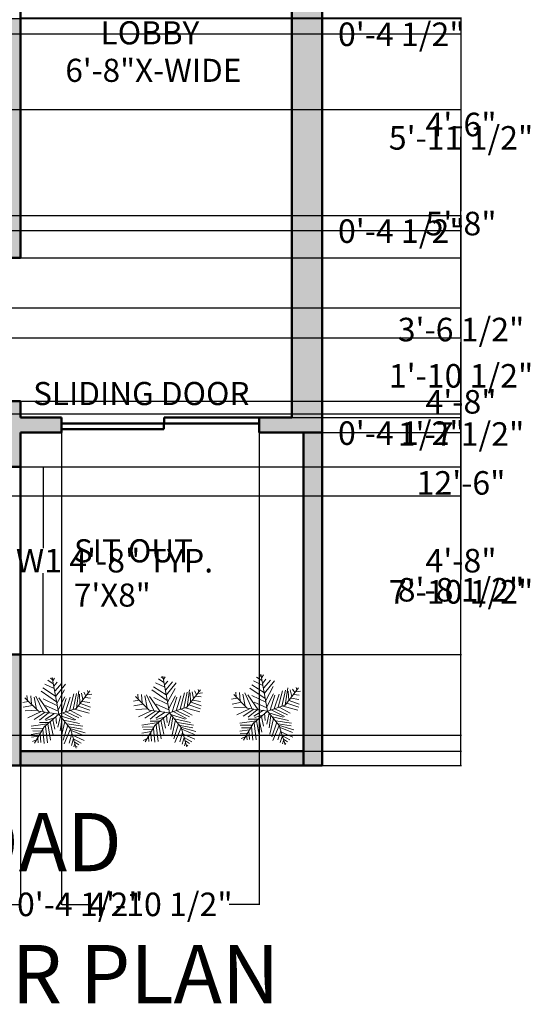
# Model space of a CAD drawing. Units: inches. Extents: x 48 to 822, y -191 to 651.
# Tile 4 of 13: x 659 to 810, y -191 to 101. Entities that reach past the tile are written whole.
import ezdxf

# ---------------------------------------------------------------- set-up
doc = ezdxf.new("R2010")
doc.units = ezdxf.units.IN
doc.header["$MEASUREMENT"] = 0
doc.layers.get('0').update_dxf_attribs({"color": 254})
for name, color, linetype, lineweight in [('A-ANNO-DIMS', 2, 'Continuous', 18), ('A-ANNO-TEXT', 3, 'Continuous', 25), ('A-AREA-IDEN', 7, 'Continuous', 25), ('A-FLOR-PATT', 252, 'Continuous', 13), ('A-WALL', 7, 'Continuous', 50), ('A-WALL-PATT', 8, 'Continuous', 13), ('L-PLNT', 103, 'Continuous', 18)]:
    doc.layers.add(name, color=color, linetype=linetype, lineweight=lineweight)
doc.styles.get("Standard").update_dxf_attribs({"font": 'arial.ttf'})
doc.dimstyles.get("Standard").update_dxf_attribs({"dimtxt": 7, "dimasz": 0.18, "dimexe": 0.18, "dimexo": 0.0625, "dimgap": 0.09, "dimtad": 0, "dimtih": 1, "dimtoh": 1, "dimzin": 0, "dimdsep": 46, "dimlunit": 3, "dimtxsty": 'Standard', "dimcen": 0.09, "dimadec": 0, "dimazin": 0, "dimtfac": 1, "dimtofl": 0, "dimtmove": 0, "dimatfit": 3, "dimfxl": 1, "dimtolj": 1, "dimtzin": 0, "dimarcsym": 0})

# ---------------------------------------------------------------- blocks, each defined once
blk = doc.blocks.new('*U15')
for p, q in [((-7.288, 39.707), (-21.778, 46.673)), ((-8.737, 47.138), (-17.069, 52.711)), ((-10.186, 53.64), (-13.084, 55.962)), ((0, 0), (-10.5, 57)), ((-9.099, 51.782), (-6.563, 55.962)), ((-7.65, 43.423), (-2.578, 49.46)), ((-5.839, 35.992), (4.667, 48.067)), ((-5.114, 27.632), (10.463, 46.673)), ((-3.665, 19.273), (-27.574, 35.527)), ((-5.114, 28.097), (-24.676, 40.636)), ((-2.941, 16.486), (8.652, 37.85)), ((16.259, 5.805), (23.142, 31.348)), ((22.055, 7.198), (27.489, 32.277)), ((27, 9), (48, 36)), ((27.127, 9.056), (31.112, 35.992)), ((31.836, 30.883), (32.561, 16.486)), ((35.096, 32.741), (37.27, 22.524)), ((38.719, 34.134), (41.979, 28.561)), ((43.791, 29.954), (51.036, 30.883)), ((44.153, 36.456), (45.239, 32.741)), ((-47.498, 19.737), (-55.83, 18.344)), ((-31.5, 4.5), (-52.5, 25.5)), ((-48.585, 21.131), (-49.309, 29.026)), ((-43.513, 28.561), (-42.427, 15.558)), ((-38.442, 26.239), (-34.819, 7.663)), ((-35.544, 28.097), (-24.314, 3.947)), ((-14.533, 2.09), (-30.834, 25.31)), ((-24.314, 23.917), (-2.941, 13.7)), ((-1.129, 6.734), (9.014, 26.704)), ((3.942, 1.625), (11.187, 24.381)), ((10.101, 3.483), (17.708, 26.239)), ((33.285, 16.486), (48.862, 10.913)), ((36.183, 19.737), (48.137, 17.88)), ((40.53, 25.775), (48.862, 24.846)), ((-40.615, 13.7), (-55.105, 10.913)), ((-33.37, 6.269), (-52.207, 5.34)), ((-28.299, 3.483), (-47.86, -5.805)), ((-21.416, 3.018), (-38.079, -8.128)), ((0, 0), (-31.5, 4.5)), ((-15.982, 2.09), (-30.11, -9.521)), ((0, 0), (-22.5, -19.5)), ((-6.563, 1.161), (-21.416, -8.128)), ((-20.691, 13.7), (-1.129, 4.876)), ((0, 0), (27, 9)), ((0, 0), (18, -22.5)), ((6.478, 1.625), (26.04, -8.592)), ((11.187, 3.483), (30.749, -5.805)), ((18.07, 5.805), (35.096, -3.483)), ((24.229, 7.663), (46.688, 1.625)), ((29.662, 12.307), (48.137, 6.269)), ((-17.431, -15.094), (-42.789, -18.809)), ((-15.257, -12.772), (-30.11, -12.772)), ((-6.563, -5.805), (-19.967, -9.985)), ((-17.069, -15.094), (-12.721, -40.172)), ((-13.446, -11.378), (-8.737, -32.741)), ((-9.461, -8.592), (-6.201, -23.453)), ((-4.752, -3.483), (-3.665, -14.629)), ((2.493, -3.019), (-1.491, -20.202)), ((1.769, -2.555), (24.229, -9.521)), ((5.029, -6.27), (2.131, -25.775)), ((9.014, -11.378), (3.58, -35.992)), ((7.565, -9.056), (32.198, -14.629)), ((12.274, -15.094), (36.907, -18.809)), ((-28.299, -29.026), (-42.789, -31.348)), ((-24.314, -21.596), (-42.427, -22.06)), ((-26.849, -26.24), (-40.253, -25.775)), ((-22.5, -19.5), (-37.5, -45)), ((-25.038, -23.918), (-22.865, -45.281)), ((-20.691, -18.345), (-17.793, -44.352)), ((14.085, -16.951), (6.478, -40.172)), ((18.07, -22.524), (8.289, -45.745)), ((20.244, -30.419), (15.897, -44.816)), ((16.259, -19.738), (36.183, -22.989)), ((18, -22.5), (27, -52.5)), ((18.433, -22.524), (40.53, -29.026)), ((19.157, -25.311), (38.719, -33.206)), ((-30.834, -34.135), (-42.427, -35.528)), ((-34.457, -39.708), (-40.978, -42.494)), ((-32.646, -36.921), (-31.921, -44.352)), ((-29.023, -30.884), (-27.936, -43.887)), ((22.78, -37.85), (19.519, -48.532)), ((21.331, -32.741), (39.081, -40.636)), ((22.78, -38.314), (34.372, -44.816)), ((24.591, -45.745), (23.142, -50.854)), ((24.591, -43.423), (30.749, -47.603)), ((26.764, -49.925), (28.213, -50.854))]:
    blk.add_line(p, q)
blk = doc.blocks.new('*D28')
at = {"layer": 'A-ANNO-DIMS', "color": 0, "lineweight": -2, "transparency": 16777216}
for p, q in [((657.56, -31.5), (666.06, -31.5)), ((665.88, -31.68), (665.88, -55.7)), ((665.88, -87.15), (665.88, -63.13)), ((657.56, -87.33), (666.06, -87.33))]:
    blk.add_line(p, q, dxfattribs=at)
at = {"layer": 'A-ANNO-DIMS', "color": 0, "transparency": 16777216}
for points in [[(665.85, -31.68), (665.91, -31.68), (665.88, -31.5)], [(665.85, -87.15), (665.91, -87.15), (665.88, -87.33)]]:
    blk.add_solid(points, dxfattribs=at)
at = {"layer": 'Defpoints', "color": 0, "transparency": 16777216}
for p in [(657.5, -31.5), (665.88, -31.5), (657.5, -87.33)]:
    blk.add_point(p, dxfattribs=at)
at = {"layer": 'A-ANNO-DIMS', "color": 0, "transparency": 16777216, "insert": (665.88, -59.42), "char_height": 7, "attachment_point": 5}
blk.add_mtext('\\A1;WINDOW W1 4\'-8" TYP.', dxfattribs=at)
blk = doc.blocks.new('*D86')
at = {"layer": 'A-ANNO-DIMS', "color": 0, "lineweight": -2, "transparency": 16777216}
for p, q in [((361.01, 74.69), (790.04, 74.69)), ((789.86, 74.51), (789.86, 44.42)), ((789.86, 7.02), (789.86, 37.1)), ((361.01, 6.84), (790.04, 6.84))]:
    blk.add_line(p, q, dxfattribs=at)
at = {"layer": 'A-ANNO-DIMS', "color": 0, "transparency": 16777216}
for points in [[(789.83, 74.51), (789.89, 74.51), (789.86, 74.69)], [(789.83, 7.02), (789.89, 7.02), (789.86, 6.84)]]:
    blk.add_solid(points, dxfattribs=at)
at = {"layer": 'Defpoints', "color": 0, "transparency": 16777216}
for p in [(360.95, 74.69), (360.95, 6.84), (789.86, 6.84)]:
    blk.add_point(p, dxfattribs=at)
at = {"layer": 'A-ANNO-DIMS', "color": 0, "transparency": 16777216, "insert": (789.86, 40.76), "char_height": 7, "attachment_point": 5}
blk.add_mtext('\\A1;5\'-8"', dxfattribs=at)
blk = doc.blocks.new('*D87')
at = {"layer": 'A-ANNO-DIMS', "color": 0, "lineweight": -2, "transparency": 16777216}
for p, q in [((361.01, 6.84), (790.04, 6.84)), ((789.86, 6.66), (789.86, -0.78)), ((789.86, -15.63), (789.86, -8.2)), ((361.01, -15.81), (790.04, -15.81))]:
    blk.add_line(p, q, dxfattribs=at)
at = {"layer": 'A-ANNO-DIMS', "color": 0, "transparency": 16777216}
for points in [[(789.83, 6.66), (789.89, 6.66), (789.86, 6.84)], [(789.83, -15.63), (789.89, -15.63), (789.86, -15.81)]]:
    blk.add_solid(points, dxfattribs=at)
at = {"layer": 'Defpoints', "color": 0, "transparency": 16777216}
for p in [(360.95, 6.84), (360.95, -15.81), (789.86, -15.81)]:
    blk.add_point(p, dxfattribs=at)
at = {"layer": 'A-ANNO-DIMS', "color": 0, "transparency": 16777216, "insert": (789.86, -4.49), "char_height": 7, "attachment_point": 5}
blk.add_mtext('\\A1;1\'-10 1/2"', dxfattribs=at)
blk = doc.blocks.new('*D88')
at = {"layer": 'A-ANNO-DIMS', "color": 0, "lineweight": -2, "transparency": 16777216}
for p, q in [((361.01, -15.81), (790.04, -15.81)), ((789.86, -15.99), (789.86, -64.35)), ((789.86, -120.13), (789.86, -71.77)), ((365.51, -120.31), (790.04, -120.31))]:
    blk.add_line(p, q, dxfattribs=at)
at = {"layer": 'A-ANNO-DIMS', "color": 0, "transparency": 16777216}
for points in [[(789.83, -15.99), (789.89, -15.99), (789.86, -15.81)], [(789.83, -120.13), (789.89, -120.13), (789.86, -120.31)]]:
    blk.add_solid(points, dxfattribs=at)
at = {"layer": 'Defpoints', "color": 0, "transparency": 16777216}
for p in [(360.95, -15.81), (365.45, -120.31), (789.86, -120.31)]:
    blk.add_point(p, dxfattribs=at)
at = {"layer": 'A-ANNO-DIMS', "color": 0, "transparency": 16777216, "insert": (789.86, -68.06), "char_height": 7, "attachment_point": 5}
blk.add_mtext('\\A1;8\'-8 1/2"', dxfattribs=at)
blk = doc.blocks.new('*D93')
at = {"layer": 'A-ANNO-DIMS', "color": 0, "lineweight": -2, "transparency": 16777216}
for p, q in [((271.51, 15.7), (790.04, 15.7)), ((789.86, 15.52), (789.86, -8.55)), ((789.86, -39.95), (789.86, -15.88)), ((271.51, -40.13), (790.04, -40.13))]:
    blk.add_line(p, q, dxfattribs=at)
at = {"layer": 'A-ANNO-DIMS', "color": 0, "transparency": 16777216}
for points in [[(789.83, 15.52), (789.89, 15.52), (789.86, 15.7)], [(789.83, -39.95), (789.89, -39.95), (789.86, -40.13)]]:
    blk.add_solid(points, dxfattribs=at)
at = {"layer": 'Defpoints', "color": 0, "transparency": 16777216}
for p in [(271.45, 15.7), (271.45, -40.13), (789.86, -40.13)]:
    blk.add_point(p, dxfattribs=at)
at = {"layer": 'A-ANNO-DIMS', "color": 0, "transparency": 16777216, "insert": (789.86, -12.22), "char_height": 7, "attachment_point": 5}
blk.add_mtext('\\A1;4\'-8"', dxfattribs=at)
blk = doc.blocks.new('*D102')
at = {"layer": 'A-ANNO-DIMS', "color": 0, "lineweight": -2, "transparency": 16777216}
for p, q in [((654.61, -111.38), (654.61, -161.74)), ((659.11, -120.38), (659.11, -161.74)), ((654.79, -161.56), (658.93, -161.56)), ((659.11, -161.56), (659.29, -161.56))]:
    blk.add_line(p, q, dxfattribs=at)
at = {"layer": 'A-ANNO-DIMS', "color": 0, "transparency": 16777216}
for points in [[(654.79, -161.53), (654.79, -161.59), (654.61, -161.56)], [(658.93, -161.53), (658.93, -161.59), (659.11, -161.56)]]:
    blk.add_solid(points, dxfattribs=at)
at = {"layer": 'Defpoints', "color": 0, "transparency": 16777216}
for p in [(654.61, -111.31), (659.11, -120.31), (659.11, -161.56)]:
    blk.add_point(p, dxfattribs=at)
at = {"layer": 'A-ANNO-DIMS', "color": 0, "transparency": 16777216, "insert": (676.84, -161.56), "char_height": 7, "attachment_point": 5}
blk.add_mtext('\\A1;0\'-4 1/2"', dxfattribs=at)
blk = doc.blocks.new('*D104')
at = {"layer": 'A-ANNO-DIMS', "color": 0, "lineweight": -2, "transparency": 16777216}
for p, q in [((671.27, -21.41), (671.27, -161.74)), ((729.97, -21.41), (729.97, -161.74)), ((671.45, -161.56), (680.21, -161.56)), ((729.79, -161.56), (721.03, -161.56))]:
    blk.add_line(p, q, dxfattribs=at)
at = {"layer": 'A-ANNO-DIMS', "color": 0, "transparency": 16777216}
for points in [[(671.45, -161.53), (671.45, -161.59), (671.27, -161.56)], [(729.79, -161.53), (729.79, -161.59), (729.97, -161.56)]]:
    blk.add_solid(points, dxfattribs=at)
at = {"layer": 'Defpoints', "color": 0, "transparency": 16777216}
for p in [(671.27, -21.34), (729.97, -21.34), (729.97, -161.56)]:
    blk.add_point(p, dxfattribs=at)
at = {"layer": 'A-ANNO-DIMS', "color": 0, "transparency": 16777216, "insert": (700.62, -161.56), "char_height": 7, "attachment_point": 5}
blk.add_mtext('\\A1;4\'-10 1/2"', dxfattribs=at)
blk = doc.blocks.new('*D114')
at = {"layer": 'A-ANNO-DIMS', "color": 0, "lineweight": -2, "transparency": 16777216}
for p, q in [((517.67, 101.69), (790.04, 101.69)), ((789.86, 101.51), (789.86, 97.37)), ((517.67, 97.19), (790.04, 97.19)), ((789.86, 97.01), (789.68, 97.01)), ((789.86, 97.19), (789.86, 97.01))]:
    blk.add_line(p, q, dxfattribs=at)
at = {"layer": 'A-ANNO-DIMS', "color": 0, "transparency": 16777216}
for points in [[(789.83, 101.51), (789.89, 101.51), (789.86, 101.69)], [(789.83, 97.37), (789.89, 97.37), (789.86, 97.19)]]:
    blk.add_solid(points, dxfattribs=at)
at = {"layer": 'Defpoints', "color": 0, "transparency": 16777216}
for p in [(517.61, 101.69), (517.61, 97.19), (789.86, 97.19)]:
    blk.add_point(p, dxfattribs=at)
at = {"layer": 'A-ANNO-DIMS', "color": 0, "transparency": 16777216, "insert": (772.13, 97.01), "char_height": 7, "attachment_point": 5}
blk.add_mtext('\\A1;0\'-4 1/2"', dxfattribs=at)
blk = doc.blocks.new('*D115')
at = {"layer": 'A-ANNO-DIMS', "color": 0, "lineweight": -2, "transparency": 16777216}
for p, q in [((517.67, 97.19), (790.04, 97.19)), ((789.86, 97.01), (789.86, 73.85)), ((789.86, 43.37), (789.86, 66.52)), ((517.67, 43.19), (790.04, 43.19))]:
    blk.add_line(p, q, dxfattribs=at)
at = {"layer": 'A-ANNO-DIMS', "color": 0, "transparency": 16777216}
for points in [[(789.83, 97.01), (789.89, 97.01), (789.86, 97.19)], [(789.83, 43.37), (789.89, 43.37), (789.86, 43.19)]]:
    blk.add_solid(points, dxfattribs=at)
at = {"layer": 'Defpoints', "color": 0, "transparency": 16777216}
for p in [(517.61, 97.19), (517.61, 43.19), (789.86, 43.19)]:
    blk.add_point(p, dxfattribs=at)
at = {"layer": 'A-ANNO-DIMS', "color": 0, "transparency": 16777216, "insert": (789.86, 70.19), "char_height": 7, "attachment_point": 5}
blk.add_mtext('\\A1;4\'-6"', dxfattribs=at)
blk = doc.blocks.new('*D116')
at = {"layer": 'A-ANNO-DIMS', "color": 0, "lineweight": -2, "transparency": 16777216}
for p, q in [((517.67, 43.19), (790.04, 43.19)), ((789.86, 43.01), (789.86, 38.87)), ((517.67, 38.69), (790.04, 38.69)), ((789.86, 38.51), (789.68, 38.51)), ((789.86, 38.69), (789.86, 38.51))]:
    blk.add_line(p, q, dxfattribs=at)
at = {"layer": 'A-ANNO-DIMS', "color": 0, "transparency": 16777216}
for points in [[(789.83, 43.01), (789.89, 43.01), (789.86, 43.19)], [(789.83, 38.87), (789.89, 38.87), (789.86, 38.69)]]:
    blk.add_solid(points, dxfattribs=at)
at = {"layer": 'Defpoints', "color": 0, "transparency": 16777216}
for p in [(517.61, 43.19), (517.61, 38.69), (789.86, 38.69)]:
    blk.add_point(p, dxfattribs=at)
at = {"layer": 'A-ANNO-DIMS', "color": 0, "transparency": 16777216, "insert": (772.13, 38.51), "char_height": 7, "attachment_point": 5}
blk.add_mtext('\\A1;0\'-4 1/2"', dxfattribs=at)
blk = doc.blocks.new('*D117')
at = {"layer": 'A-ANNO-DIMS', "color": 0, "lineweight": -2, "transparency": 16777216}
for p, q in [((517.67, 38.69), (790.04, 38.69)), ((789.86, 38.51), (789.86, -32.65)), ((789.86, -111.13), (789.86, -39.98)), ((517.67, -111.31), (790.04, -111.31))]:
    blk.add_line(p, q, dxfattribs=at)
at = {"layer": 'A-ANNO-DIMS', "color": 0, "transparency": 16777216}
for points in [[(789.83, 38.51), (789.89, 38.51), (789.86, 38.69)], [(789.83, -111.13), (789.89, -111.13), (789.86, -111.31)]]:
    blk.add_solid(points, dxfattribs=at)
at = {"layer": 'Defpoints', "color": 0, "transparency": 16777216}
for p in [(517.61, 38.69), (517.61, -111.31), (789.86, -111.31)]:
    blk.add_point(p, dxfattribs=at)
at = {"layer": 'A-ANNO-DIMS', "color": 0, "transparency": 16777216, "insert": (789.86, -36.31), "char_height": 7, "attachment_point": 5}
blk.add_mtext('\\A1;12\'-6"', dxfattribs=at)
blk = doc.blocks.new('*D122')
at = {"layer": 'A-ANNO-DIMS', "color": 0, "lineweight": -2, "transparency": 16777216}
for p, q in [((739.67, -16.84), (790.04, -16.84)), ((789.86, -17.02), (789.86, -21.16)), ((743.17, -21.34), (790.04, -21.34)), ((789.86, -21.52), (789.68, -21.52)), ((789.86, -21.34), (789.86, -21.52))]:
    blk.add_line(p, q, dxfattribs=at)
at = {"layer": 'A-ANNO-DIMS', "color": 0, "transparency": 16777216}
for points in [[(789.83, -17.02), (789.89, -17.02), (789.86, -16.84)], [(789.83, -21.16), (789.89, -21.16), (789.86, -21.34)]]:
    blk.add_solid(points, dxfattribs=at)
at = {"layer": 'Defpoints', "color": 0, "transparency": 16777216}
for p in [(739.61, -16.84), (743.11, -21.34), (789.86, -21.34)]:
    blk.add_point(p, dxfattribs=at)
at = {"layer": 'A-ANNO-DIMS', "color": 0, "transparency": 16777216, "insert": (772.13, -21.52), "char_height": 7, "attachment_point": 5}
blk.add_mtext('\\A1;0\'-4 1/2"', dxfattribs=at)
blk = doc.blocks.new('*D123')
at = {"layer": 'A-ANNO-DIMS', "color": 0, "lineweight": -2, "transparency": 16777216}
for p, q in [((743.17, -21.34), (790.04, -21.34)), ((789.86, -21.52), (789.86, -64.98)), ((789.86, -115.85), (789.86, -72.39)), ((743.17, -116.03), (790.04, -116.03))]:
    blk.add_line(p, q, dxfattribs=at)
at = {"layer": 'A-ANNO-DIMS', "color": 0, "transparency": 16777216}
for points in [[(789.83, -21.52), (789.89, -21.52), (789.86, -21.34)], [(789.83, -115.85), (789.89, -115.85), (789.86, -116.03)]]:
    blk.add_solid(points, dxfattribs=at)
at = {"layer": 'Defpoints', "color": 0, "transparency": 16777216}
for p in [(743.11, -21.34), (743.11, -116.03), (789.86, -116.03)]:
    blk.add_point(p, dxfattribs=at)
at = {"layer": 'A-ANNO-DIMS', "color": 0, "transparency": 16777216, "insert": (789.86, -68.68), "char_height": 7, "attachment_point": 5}
blk.add_mtext('\\A1;7\'-10 1/2"', dxfattribs=at)
blk = doc.blocks.new('*D130')
at = {"layer": 'A-ANNO-DIMS', "color": 0, "lineweight": -2, "transparency": 16777216}
for p, q in [((659.17, 101.9), (790.04, 101.9)), ((789.86, 101.72), (789.86, 69.94)), ((789.86, 30.74), (789.86, 62.52)), ((659.17, 30.56), (790.04, 30.56))]:
    blk.add_line(p, q, dxfattribs=at)
at = {"layer": 'A-ANNO-DIMS', "color": 0, "transparency": 16777216}
for points in [[(789.83, 101.72), (789.89, 101.72), (789.86, 101.9)], [(789.83, 30.74), (789.89, 30.74), (789.86, 30.56)]]:
    blk.add_solid(points, dxfattribs=at)
at = {"layer": 'Defpoints', "color": 0, "transparency": 16777216}
for p in [(659.11, 101.9), (659.11, 30.56), (789.86, 30.56)]:
    blk.add_point(p, dxfattribs=at)
at = {"layer": 'A-ANNO-DIMS', "color": 0, "transparency": 16777216, "insert": (789.86, 66.23), "char_height": 7, "attachment_point": 5}
blk.add_mtext('\\A1;5\'-11 1/2"', dxfattribs=at)
blk = doc.blocks.new('*D131')
at = {"layer": 'A-ANNO-DIMS', "color": 0, "lineweight": -2, "transparency": 16777216}
for p, q in [((659.17, 30.56), (790.04, 30.56)), ((789.86, 30.38), (789.86, 12.97)), ((789.86, -11.87), (789.86, 5.54)), ((659.17, -12.05), (790.04, -12.05))]:
    blk.add_line(p, q, dxfattribs=at)
at = {"layer": 'A-ANNO-DIMS', "color": 0, "transparency": 16777216}
for points in [[(789.83, 30.38), (789.89, 30.38), (789.86, 30.56)], [(789.83, -11.87), (789.89, -11.87), (789.86, -12.05)]]:
    blk.add_solid(points, dxfattribs=at)
at = {"layer": 'Defpoints', "color": 0, "transparency": 16777216}
for p in [(659.11, 30.56), (659.11, -12.05), (789.86, -12.05)]:
    blk.add_point(p, dxfattribs=at)
at = {"layer": 'A-ANNO-DIMS', "color": 0, "transparency": 16777216, "insert": (789.86, 9.26), "char_height": 7, "attachment_point": 5}
blk.add_mtext('\\A1;3\'-6 1/2"', dxfattribs=at)
blk = doc.blocks.new('*D132')
at = {"layer": 'A-ANNO-DIMS', "color": 0, "lineweight": -2, "transparency": 16777216}
for p, q in [((659.17, -12.05), (790.04, -12.05)), ((789.86, -12.23), (789.86, -18.07)), ((789.86, -31.32), (789.86, -25.49)), ((659.17, -31.5), (790.04, -31.5))]:
    blk.add_line(p, q, dxfattribs=at)
at = {"layer": 'A-ANNO-DIMS', "color": 0, "transparency": 16777216}
for points in [[(789.83, -12.23), (789.89, -12.23), (789.86, -12.05)], [(789.83, -31.32), (789.89, -31.32), (789.86, -31.5)]]:
    blk.add_solid(points, dxfattribs=at)
at = {"layer": 'Defpoints', "color": 0, "transparency": 16777216}
for p in [(659.11, -12.05), (659.11, -31.5), (789.86, -31.5)]:
    blk.add_point(p, dxfattribs=at)
at = {"layer": 'A-ANNO-DIMS', "color": 0, "transparency": 16777216, "insert": (789.86, -21.78), "char_height": 7, "attachment_point": 5}
blk.add_mtext('\\A1;1\'-7 1/2"', dxfattribs=at)
blk = doc.blocks.new('*D133')
at = {"layer": 'A-ANNO-DIMS', "color": 0, "lineweight": -2, "transparency": 16777216}
for p, q in [((659.17, -31.5), (790.04, -31.5)), ((789.86, -31.68), (789.86, -55.75)), ((789.86, -87.15), (789.86, -63.08)), ((659.17, -87.33), (790.04, -87.33))]:
    blk.add_line(p, q, dxfattribs=at)
at = {"layer": 'A-ANNO-DIMS', "color": 0, "transparency": 16777216}
for points in [[(789.83, -31.68), (789.89, -31.68), (789.86, -31.5)], [(789.83, -87.15), (789.89, -87.15), (789.86, -87.33)]]:
    blk.add_solid(points, dxfattribs=at)
at = {"layer": 'Defpoints', "color": 0, "transparency": 16777216}
for p in [(659.11, -31.5), (659.11, -87.33), (789.86, -87.33)]:
    blk.add_point(p, dxfattribs=at)
at = {"layer": 'A-ANNO-DIMS', "color": 0, "transparency": 16777216, "insert": (789.86, -59.42), "char_height": 7, "attachment_point": 5}
blk.add_mtext('\\A1;4\'-8"', dxfattribs=at)

msp = doc.modelspace()

# ---------------------------------------------------------------- hatches: boundary and pattern name
at = {"layer": 'A-FLOR-PATT'}
h = msp.add_hatch(color=256, dxfattribs=at)
h.dxf.hatch_style = 1
h.paths.add_polyline_path([(743.11, -116.025), (659.11, -116.025), (659.11, -120.313), (743.11, -120.313)])
at = {"layer": 'A-WALL-PATT'}
h = msp.add_hatch(color=256, dxfattribs=at)
h.dxf.hatch_style = 1
h.paths.add_polyline_path([(614.11, 432.437), (609.61, 432.437), (609.61, 376.187), (535.284, 376.187), (535.284, 371.687), (547.61, 371.687), (547.61, 359.12), (552.11, 359.12), (552.11, 371.687), (609.61, 371.687), (609.61, 335.687), (614.11, 335.687)], flags=17)
h.paths.add_polyline_path([(614.11, 434.687), (609.61, 434.687), (609.61, 432.437), (614.11, 432.437)], flags=17)
h.paths.add_polyline_path([(573.934, 434.687), (517.61, 434.687), (517.61, 590.687), (650.61, 590.687), (650.61, 585.522), (655.11, 585.522), (655.11, 590.687), (739.61, 590.687), (739.61, 548.687), (655.11, 548.687), (655.11, 550.72), (650.61, 550.72), (650.61, 458.608), (655.11, 458.608), (655.11, 544.187), (739.61, 544.187), (739.61, 434.541), (650.61, 434.541), (650.61, 430.041), (739.61, 430.041), (739.61, -16.844), (729.973, -16.844), (729.973, -21.344), (748.61, -21.344), (748.61, 599.687), (508.61, 599.687), (508.61, -120.313), (543.114, -120.313), (543.114, -111.313), (517.61, -111.313), (517.61, 38.687), (607.29, 38.687), (607.29, 43.187), (517.61, 43.187), (517.61, 97.187), (654.61, 97.187), (654.61, 30.562), (659.11, 30.562), (659.11, 101.895), (654.61, 101.895), (654.61, 101.687), (517.61, 101.687), (517.61, 221.687), (654.61, 221.687), (654.61, 218.066), (659.11, 218.066), (659.11, 226.187), (517.61, 226.187), (517.61, 295.187), (614.11, 295.187), (648.087, 295.187), (661.07, 295.187), (661.07, 299.687), (614.11, 299.687), (552.11, 299.687), (552.11, 341.37), (547.61, 341.37), (547.61, 299.687), (517.61, 299.687), (517.61, 371.687), (517.534, 371.687), (517.534, 376.187), (517.61, 430.187), (573.934, 430.187)])
h.paths.add_polyline_path([(659.11, -87.328), (654.61, -87.328), (654.61, -111.313), (598.94, -111.313), (598.94, -120.313), (659.11, -120.313)], flags=0)
h.paths.add_polyline_path([(671.266, -16.844), (659.11, -16.844), (659.11, -12.05), (654.61, -12.05), (654.61, -31.502), (659.11, -31.502), (659.11, -21.344), (671.266, -21.344)], flags=17)
h.paths.add_polyline_path([(606.11, 97.187), (601.61, 97.187), (601.61, 75.902), (606.11, 75.902)], flags=17)
h.paths.add_polyline_path([(659.11, 169.875), (654.61, 169.875), (654.61, 157.721), (659.11, 157.721)], flags=17)
h = msp.add_hatch(color=256, dxfattribs=at)
h.dxf.hatch_style = 1
h.paths.add_polyline_path([(365.451, 74.687), (360.951, 74.687), (360.951, -120.313), (365.451, -120.313)])
h.paths.add_polyline_path([(275.951, -115.813), (129.951, -115.813), (129.951, -67.813), (125.451, -67.813), (125.451, -120.313), (275.951, -120.313)])
h.paths.add_polyline_path([(748.61, -21.344), (743.11, -21.344), (743.11, -120.313), (748.61, -120.313)])
h = msp.add_hatch(color=256, dxfattribs=at)
h.dxf.hatch_style = 1
h.paths.add_polyline_path([(659.11, -87.328), (654.61, -87.328), (654.61, -111.313), (598.94, -111.313), (598.94, -120.313), (659.11, -120.313)])

# ---------------------------------------------------------------- linework, layer by layer
at = {"layer": 'A-WALL'}
for p, q in [((748.61, 599.687), (748.61, -120.313)), ((739.61, 430.041), (739.61, -16.844)), ((659.11, 30.562), (659.11, 169.875)), ((654.61, 30.562), (659.11, 30.562)), ((654.61, -12.05), (659.11, -12.05)), ((659.11, -16.844), (659.11, -12.05)), ((659.11, -16.844), (671.266, -16.844)), ((671.266, -16.844), (671.266, -21.344)), ((729.973, -16.844), (701.709, -16.844)), ((701.709, -16.844), (701.709, -18.609)), ((729.973, -16.844), (729.973, -21.344)), ((729.973, -16.844), (739.61, -16.844)), ((671.266, -18.609), (701.644, -18.609)), ((701.644, -20.373), (671.266, -20.373)), ((701.644, -18.609), (701.644, -20.373)), ((701.709, -18.609), (729.973, -18.609)), ((659.11, -120.313), (659.11, -21.344)), ((659.11, -21.344), (671.266, -21.344)), ((729.973, -21.344), (748.61, -21.344)), ((743.11, -120.313), (743.11, -21.344)), ((659.11, -31.502), (654.61, -31.502)), ((659.11, -87.328), (659.11, -31.502)), ((654.61, -87.328), (659.11, -87.328)), ((743.11, -116.025), (659.11, -116.025)), ((659.11, -120.313), (508.61, -120.313)), ((659.11, -120.313), (743.11, -120.313)), ((748.61, -120.313), (743.11, -120.313))]:
    msp.add_line(p, q, dxfattribs=at)

# ---------------------------------------------------------------- block references
at = {"layer": 'L-PLNT', "xscale": 0.1917994770544849, "yscale": 0.1917994770544849, "zscale": 0.1917994770544849}
for p in [(732.466, -104.112), (670.491, -105.038), (703.344, -104.665)]:
    msp.add_blockref('*U15', p, dxfattribs=at)

# ---------------------------------------------------------------- texts
at = {"layer": 'A-ANNO-TEXT'}
for s, height, p in [('MAIN ROAD', 17.3215, (563.17, -151.725)), ('FIRST FLOOR PLAN', 17.32149, (527.002, -190.95))]:
    msp.add_text(s, height=height, dxfattribs=at).set_placement(p)
at = {"layer": 'A-AREA-IDEN'}
for s, height, p in [('LOBBY', 6.866, (682.87, 94.016)), ('6\'-8"X-WIDE', 6.86603, (672.423, 82.861)), ('SLIDING DOOR', 6.86603, (662.851, -13.179)), ('SIT OUT', 6.866, (674.957, -59.919)), ('7\'X8"', 6.866, (674.957, -73.078))]:
    msp.add_text(s, height=height, dxfattribs=at).set_placement(p)

# ---------------------------------------------------------------- dimensions: what is measured, and where the dimension line sits
at = {"layer": 'A-ANNO-DIMS'}
for base, p1, p2, picture, middle in [((789.86, 97.187), (517.61, 101.687), (517.61, 97.187), '*D114', (772.131, 97.007)), ((789.86, 30.562), (659.11, 101.895), (659.11, 30.562), '*D130', (789.86, 66.229)), ((789.86, 43.187), (517.61, 97.187), (517.61, 43.187), '*D115', (789.86, 70.187)), ((789.86, 6.835), (360.951, 74.687), (360.951, 6.835), '*D86', (789.86, 40.761)), ((789.86, 38.687), (517.61, 43.187), (517.61, 38.687), '*D116', (772.131, 38.507)), ((789.86, -111.313), (517.61, 38.687), (517.61, -111.313), '*D117', (789.86, -36.313)), ((789.86, -12.05), (659.11, 30.562), (659.11, -12.05), '*D131', (789.86, 9.256)), ((789.86, -40.13), (271.451, 15.696), (271.451, -40.13), '*D93', (789.86, -12.217)), ((789.86, -15.813), (360.951, 6.835), (360.951, -15.813), '*D87', (789.86, -4.489)), ((789.86, -31.502), (659.11, -12.05), (659.11, -31.502), '*D132', (789.86, -21.776)), ((789.86, -21.344), (739.61, -16.844), (743.11, -21.344), '*D122', (772.131, -21.524)), ((789.86, -120.313), (360.951, -15.813), (365.451, -120.313), '*D88', (789.86, -68.063)), ((789.86, -116.025), (743.11, -21.344), (743.11, -116.025), '*D123', (789.86, -68.685)), ((789.86, -87.328), (659.11, -31.502), (659.11, -87.328), '*D133', (789.86, -59.415))]:
    dim = msp.add_linear_dim(base=base, p1=p1, p2=p2, angle=90, dimstyle='Standard', override={"dimdec": 1, "dimlfac": 1, "dimrnd": 0, "dimzin": 1, "dimdsep": 46, "dimlunit": 4, "dimfrac": 2}, dxfattribs=at)
    dim.commit()
    dim.dimension.update_dxf_attribs({"geometry": picture, "text_midpoint": middle})
for base, p1, p2, picture, middle in [((729.973, -161.563), (671.266, -21.344), (729.973, -21.344), '*D104', (700.619, -161.563)), ((659.11, -161.563), (654.61, -111.313), (659.11, -120.313), '*D102', (676.84, -161.563))]:
    dim = msp.add_linear_dim(base=base, p1=p1, p2=p2, dimstyle='Standard', override={"dimdec": 1, "dimlfac": 1, "dimrnd": 0, "dimzin": 1, "dimdsep": 46, "dimlunit": 4, "dimfrac": 2}, dxfattribs=at)
    dim.commit()
    dim.dimension.update_dxf_attribs({"geometry": picture, "text_midpoint": middle})
dim = msp.add_linear_dim(base=(665.875, -31.502), p1=(657.501, -87.328), p2=(657.501, -31.502), angle=90, text='WINDOW W1 <> TYP.', dimstyle='Standard', override={"dimdec": 1, "dimlfac": 1, "dimrnd": 0, "dimzin": 1, "dimdsep": 46, "dimlunit": 4, "dimfrac": 2}, dxfattribs=at)
dim.commit()
dim.dimension.update_dxf_attribs({"geometry": '*D28', "text_midpoint": (665.875, -59.415)})

doc.saveas('drawing.dxf')
